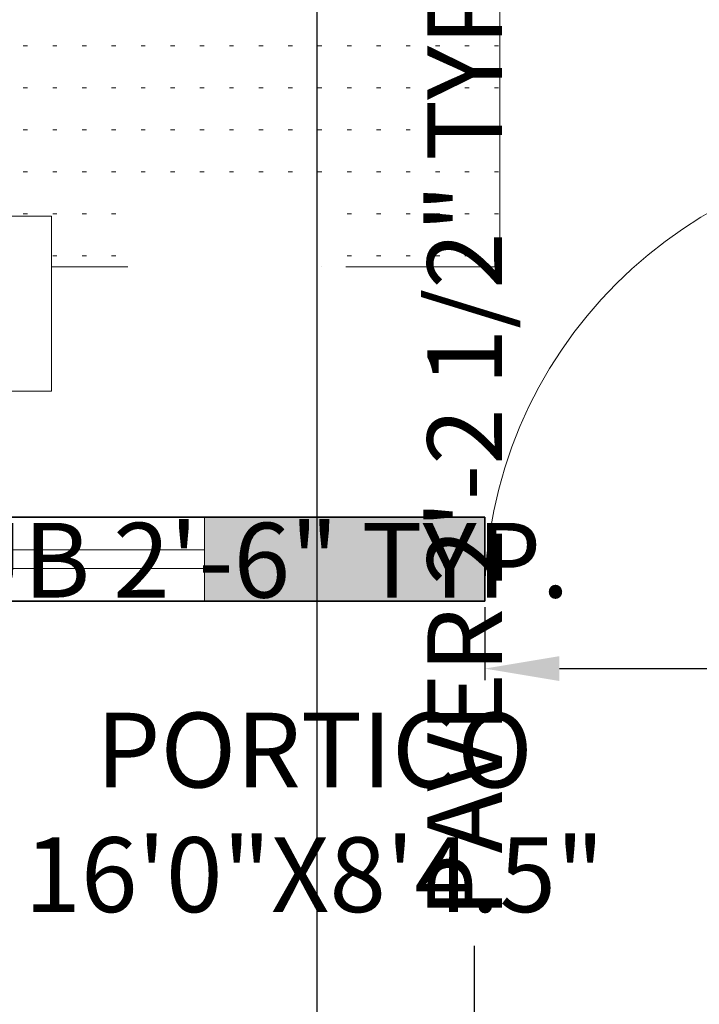
# Model space of a CAD drawing. Units: inches. Extents: x 2408 to 5087, y 2429 to 5085.
# Tile 5 of 12: x 2564 to 2636, y 2570 to 2676. Entities that reach past the tile are written whole.
import ezdxf

# ---------------------------------------------------------------- set-up
doc = ezdxf.new("R2010")
doc.units = ezdxf.units.IN
for name, color, linetype, lineweight in [('A-ANNO-DIMS', 2, 'Continuous', 18), ('A-AREA-IDEN', 6, 'Continuous', 18), ('A-DOOR', 3, 'Continuous', 18), ('A-FLOR-PATT', 8, 'Continuous', 13), ('A-FURN', 72, 'Continuous', 18), ('A-GLAZ', 4, 'Continuous', 18), ('A-WALL', 7, 'Continuous', 35), ('A-WALL-PATT', 252, 'Continuous', 13)]:
    doc.layers.add(name, color=color, linetype=linetype, lineweight=lineweight)
doc.styles.get("Standard").update_dxf_attribs({"font": 'arial.ttf'})
doc.dimstyles.new('ISO-25', dxfattribs={"dimtxt": 8, "dimasz": 8, "dimexe": 1.25, "dimexo": 0.625, "dimtad": 0, "dimdec": 1, "dimlunit": 4, "dimtxsty": 'Standard', "dimcen": 2.5, "dimadec": 0, "dimazin": 0, "dimtfac": 1, "dimtdec": 1, "dimtmove": 0, "dimatfit": 3, "dimfxl": 1, "dimarcsym": 0})

# ---------------------------------------------------------------- blocks, each defined once
blk = doc.blocks.new('door')
blk.add_lwpolyline([(2353.246, 2862.233), (2353.246, 2898.06), (2351.474, 2898.06), (2351.474, 2862.233), (2353.246, 2862.233)])
blk.add_arc((2353.246, 2862.233), 35.827, 90, 180)
blk = doc.blocks.new('Clinicians and patient chairs 25_dwgmodels.com')
at = {"color": 0}
for points in [[(-289.5, -1.5, 0, 0, 0), (-290.1, -3.2, 4.37, 4.37, 0)], [(-287.1, -0.3, 0, 0, 0), (-289.5, -1.5, 4.37, 4.37, 0)], [(-287.1, -0.3, 0, 0, 0), (-265.1, -0.9, 4.37, 4.37, 0)], [(-265.1, -0.9, 0, 0, 0), (-198.5, -0.4, 4.37, 4.37, 0)], [(-198.5, -0.4, 0, 0, 0), (-92.3, -0.3, 4.37, 4.37, 0)], [(-92.3, -0.3, 0, 0, 0), (0, 0, 4.37, 4.37, 0)], [(92.3, -0.3, 0, 0, 0), (0, 0, 4.37, 4.37, 0)], [(198.5, -0.4, 0, 0, 0), (92.3, -0.3, 4.37, 4.37, 0)], [(265.7, -0.9, 0, 0, 0), (198.5, -0.4, 4.37, 4.37, 0)], [(287.7, -0.3, 0, 0, 0), (265.7, -0.9, 4.37, 4.37, 0)], [(287.7, -0.3, 0, 0, 0), (290.1, -1.5, 4.37, 4.37, 0)], [(290.1, -1.5, 0, 0, 0), (290.7, -3.2, 4.37, 4.37, 0)], [(-371.8, -16.6, 0, 0, 0), (-369.1, -9.1, 4.37, 4.37, 0)], [(-371.8, -16.5, 0, 0, 0), (-369.8, -11, 4.37, 4.37, 0)], [(-371.8, -16.6, 0, 0, 0), (-371.8, -705.5, 4.37, 4.37, 0)], [(-371.8, -16.6, 0, 0, 0), (-371.8, -705.5, 4.37, 4.37, 0)], [(-369.8, -8.3, 0, 0, 0), (-369.7, -10.5, 4.37, 4.37, 0)], [(-369.8, -8.3, 0, 0, 0), (-369.8, -9.6, 4.37, 4.37, 0)], [(-369.8, -8.3, 0, 0, 0), (-367.7, -8.5, 4.37, 4.37, 0)], [(-369.8, -11, 0, 0, 0), (-369.8, -11, 4.37, 4.37, 0)], [(-369.8, -11, 0, 0, 0), (-369.8, -11, 4.37, 4.37, 0)], [(-369.8, -11, 0, 0, 0), (-369.8, -11, 4.37, 4.37, 0)], [(-369.7, -10.5, 0, 0, 0), (-369.6, -10.6, 4.37, 4.37, 0)], [(-369.1, -9.1, 0, 0, 0), (-361.2, -6.5, 4.37, 4.37, 0)], [(-367.7, -8.5, 0, 0, 0), (-367.6, -8.6, 4.37, 4.37, 0)], [(-367.7, -8.5, 0, 0, 0), (-367.6, -8.6, 4.37, 4.37, 0)], [(-361.2, -6.5, 0, 0, 0), (-367.2, -8.4, 4.37, 4.37, 0)], [(-367.2, -8.4, 0, 0, 0), (-367.2, -8.4, 4.37, 4.37, 0)], [(-367.2, -8.5, 0, 0, 0), (-367.2, -8.4, 4.37, 4.37, 0)], [(-299.5, -6.5, 0, 0, 0), (-361.2, -6.5, 4.37, 4.37, 0)], [(-299.5, -6.5, 0, 0, 0), (-294.7, -8, 4.37, 4.37, 0)], [(-299.5, -6.5, 0, 0, 0), (-294.7, -8.1, 4.37, 4.37, 0)], [(-294.8, -48.3, 0, 0, 0), (-294.8, -31.9, 4.37, 4.37, 0)], [(-294.7, -6.7, 0, 0, 0), (-291.8, -2.6, 4.37, 4.37, 0)], [(-294.8, -31.9, 0, 0, 0), (-294.7, -6.7, 4.37, 4.37, 0)], [(-294.7, -29.9, 0, 0, 0), (-294.5, -13.6, 4.37, 4.37, 0)], [(-294.7, -29.9, 0, 0, 0), (-294.8, -31.9, 4.37, 4.37, 0)], [(-291.8, -2.6, 0, 0, 0), (-290.1, -3.2, 4.37, 4.37, 0)], [(-289.7, -10.8, 0, 0, 0), (-290.1, -3.2, 4.37, 4.37, 0)], [(-290.1, -51.3, 0, 0, 0), (-290, -30, 4.37, 4.37, 0)], [(-290, -30, 0, 0, 0), (-289.7, -10.8, 4.37, 4.37, 0)], [(290.3, -10.8, 0, 0, 0), (290.7, -3.2, 4.37, 4.37, 0)], [(290.7, -30, 0, 0, 0), (290.3, -10.8, 4.37, 4.37, 0)], [(292.4, -2.6, 0, 0, 0), (290.7, -3.2, 4.37, 4.37, 0)], [(290.7, -51.3, 0, 0, 0), (290.7, -30, 4.37, 4.37, 0)], [(295.4, -6.7, 0, 0, 0), (292.4, -2.6, 4.37, 4.37, 0)], [(295.4, -29.9, 0, 0, 0), (295.1, -13.6, 4.37, 4.37, 0)], [(299.5, -6.5, 0, 0, 0), (295.4, -7.9, 4.37, 4.37, 0)], [(299.5, -6.5, 0, 0, 0), (295.4, -7.8, 4.37, 4.37, 0)], [(295.4, -31.9, 0, 0, 0), (295.4, -6.7, 4.37, 4.37, 0)], [(295.4, -29.9, 0, 0, 0), (295.4, -31.9, 4.37, 4.37, 0)], [(295.4, -31.9, 0, 0, 0), (295.4, -48.3, 4.37, 4.37, 0)], [(299.5, -6.5, 0, 0, 0), (361.2, -6.5, 4.37, 4.37, 0)], [(369.1, -9.1, 0, 0, 0), (361.2, -6.5, 4.37, 4.37, 0)], [(369.1, -9.1, 0, 0, 0), (361.2, -6.5, 4.37, 4.37, 0)], [(361.2, -6.6, 0, 0, 0), (367.2, -8.4, 4.37, 4.37, 0)], [(367.2, -8.4, 0, 0, 0), (367.2, -8.4, 4.37, 4.37, 0)], [(367.2, -8.5, 0, 0, 0), (367.2, -8.4, 4.37, 4.37, 0)], [(367.7, -8.5, 0, 0, 0), (367.6, -8.6, 4.37, 4.37, 0)], [(367.7, -8.5, 0, 0, 0), (367.6, -8.6, 4.37, 4.37, 0)], [(369.8, -8.3, 0, 0, 0), (367.7, -8.5, 4.37, 4.37, 0)], [(371.8, -16.6, 0, 0, 0), (369.1, -9.1, 4.37, 4.37, 0)], [(369.4, -10, 0, 0, 0), (369.4, -10, 4.37, 4.37, 0)], [(369.7, -10.5, 0, 0, 0), (369.6, -10.6, 4.37, 4.37, 0)], [(369.8, -8.3, 0, 0, 0), (369.7, -10.5, 4.37, 4.37, 0)], [(369.8, -8.3, 0, 0, 0), (369.8, -9.6, 4.37, 4.37, 0)], [(371.8, -16.5, 0, 0, 0), (369.8, -11, 4.37, 4.37, 0)], [(369.8, -11, 0, 0, 0), (369.8, -11, 4.37, 4.37, 0)], [(369.8, -11, 0, 0, 0), (369.8, -11, 4.37, 4.37, 0)], [(369.8, -11, 0, 0, 0), (369.8, -11, 4.37, 4.37, 0)], [(371.8, -16.6, 0, 0, 0), (371.8, -705.5, 4.37, 4.37, 0)], [(-371.8, -44.1, 0, 0, 0), (-371.8, -361, 4.37, 4.37, 0)], [(-294.8, -48.3, 0, 0, 0), (-294.7, -60.2, 4.37, 4.37, 0)], [(-294.7, -60.2, 0, 0, 0), (-294.7, -69.9, 4.37, 4.37, 0)], [(-290, -64.7, 0, 0, 0), (-290.1, -51.3, 4.37, 4.37, 0)], [(-290, -64.7, 0, 0, 0), (-290, -74.5, 4.37, 4.37, 0)], [(-284.2, -72.8, 0, 0, 0), (-262.5, -66.3, 4.37, 4.37, 0)], [(-276.4, -68.7, 0, 0, 0), (-280.9, -71.1, 4.37, 4.37, 0)], [(-276.4, -68.7, 0, 0, 0), (-257.9, -63.2, 4.37, 4.37, 0)], [(-262.5, -66.3, 0, 0, 0), (-233.5, -62.8, 4.37, 4.37, 0)], [(-262, -69.5, 0, 0, 0), (-233.2, -66.1, 4.37, 4.37, 0)], [(-257.9, -63.2, 0, 0, 0), (-233.1, -60.2, 4.37, 4.37, 0)], [(-233.5, -62.8, 0, 0, 0), (-96.6, -62.8, 4.37, 4.37, 0)], [(-96.6, -66, 0, 0, 0), (-233.2, -66.1, 4.37, 4.37, 0)], [(-233.1, -60.2, 0, 0, 0), (-96.5, -60.1, 4.37, 4.37, 0)], [(126.5, -62.8, 0, 0, 0), (-96.6, -62.8, 4.37, 4.37, 0)], [(126.5, -66, 0, 0, 0), (-96.6, -66, 4.37, 4.37, 0)], [(126.4, -60.1, 0, 0, 0), (-96.5, -60.1, 4.37, 4.37, 0)], [(233.6, -60.2, 0, 0, 0), (126.4, -60.1, 4.37, 4.37, 0)], [(234, -62.8, 0, 0, 0), (126.5, -62.8, 4.37, 4.37, 0)], [(126.5, -66, 0, 0, 0), (233.8, -66.1, 4.37, 4.37, 0)], [(258.5, -63.2, 0, 0, 0), (233.6, -60.2, 4.37, 4.37, 0)], [(262.5, -69.5, 0, 0, 0), (233.8, -66.1, 4.37, 4.37, 0)], [(234, -62.8, 0, 0, 0), (263.1, -66.3, 4.37, 4.37, 0)], [(277, -68.7, 0, 0, 0), (258.5, -63.2, 4.37, 4.37, 0)], [(284.7, -72.8, 0, 0, 0), (263.1, -66.3, 4.37, 4.37, 0)], [(277, -68.7, 0, 0, 0), (281.4, -71.1, 4.37, 4.37, 0)], [(290.7, -64.7, 0, 0, 0), (290.7, -51.3, 4.37, 4.37, 0)], [(290.6, -74.5, 0, 0, 0), (290.7, -64.7, 4.37, 4.37, 0)], [(295.4, -60.2, 0, 0, 0), (295.4, -48.3, 4.37, 4.37, 0)], [(295.4, -60.2, 0, 0, 0), (295.4, -69.9, 4.37, 4.37, 0)], [(371.8, -44.1, 0, 0, 0), (371.8, -361, 4.37, 4.37, 0)], [(-293, -92.7, 0, 0, 0), (-295.9, -118.4, 4.37, 4.37, 0)], [(-294.7, -69.9, 0, 0, 0), (-294.7, -86.3, 4.37, 4.37, 0)], [(-294.7, -86.3, 0, 0, 0), (-294.7, -87.6, 4.37, 4.37, 0)], [(-294.7, -87.6, 0, 0, 0), (-294.7, -87.7, 4.37, 4.37, 0)], [(-294.5, -88.2, 0, 0, 0), (-294.7, -87.7, 4.37, 4.37, 0)], [(-292.8, -91.5, 0, 0, 0), (-294.5, -88.2, 4.37, 4.37, 0)], [(-293, -92.7, 0, 0, 0), (-291.6, -83.8, 4.37, 4.37, 0)], [(-291.8, -79.4, 0, 0, 0), (-284.2, -72.8, 4.37, 4.37, 0)], [(-291.8, -79.4, 0, 0, 0), (-291.8, -84.9, 4.37, 4.37, 0)], [(-291.6, -83.8, 0, 0, 0), (-290.8, -82.4, 4.37, 4.37, 0)], [(-283.3, -75.9, 0, 0, 0), (-290.8, -82.4, 4.37, 4.37, 0)], [(-290, -74.5, 0, 0, 0), (-290, -77.9, 4.37, 4.37, 0)], [(-283.3, -75.9, 0, 0, 0), (-262, -69.5, 4.37, 4.37, 0)], [(-280.9, -71.1, 0, 0, 0), (-282.2, -72.2, 4.37, 4.37, 0)], [(262.5, -69.5, 0, 0, 0), (283.8, -75.9, 4.37, 4.37, 0)], [(281.4, -71.1, 0, 0, 0), (282.8, -72.2, 4.37, 4.37, 0)], [(283.8, -75.9, 0, 0, 0), (289.6, -80.9, 4.37, 4.37, 0)], [(284.7, -72.8, 0, 0, 0), (291.2, -78.5, 4.37, 4.37, 0)], [(289.8, -81.8, 0, 0, 0), (289.6, -80.9, 4.37, 4.37, 0)], [(289.8, -81.8, 0, 0, 0), (291.4, -92.3, 4.37, 4.37, 0)], [(290.6, -74.5, 0, 0, 0), (290.7, -78, 4.37, 4.37, 0)], [(292.4, -98.2, 0, 0, 0), (291.2, -78.5, 4.37, 4.37, 0)], [(294.4, -118.8, 0, 0, 0), (291.4, -92.3, 4.37, 4.37, 0)], [(292.1, -93.2, 0, 0, 0), (292.6, -93.1, 4.37, 4.37, 0)], [(292.3, -100.4, 0, 0, 0), (292.4, -100.3, 4.37, 4.37, 0)], [(292.4, -100.2, 0, 0, 0), (292.4, -98.2, 4.37, 4.37, 0)], [(292.8, -92.7, 0, 0, 0), (292.6, -93.1, 4.37, 4.37, 0)], [(292.8, -92.7, 0, 0, 0), (294.5, -89.3, 4.37, 4.37, 0)], [(294.5, -89.3, 0, 0, 0), (294.9, -88.5, 4.37, 4.37, 0)], [(294.9, -88.5, 0, 0, 0), (295.3, -87.6, 4.37, 4.37, 0)], [(295.4, -69.9, 0, 0, 0), (295.3, -86.3, 4.37, 4.37, 0)], [(295.3, -86.3, 0, 0, 0), (295.3, -87.8, 4.37, 4.37, 0)], [(-295.9, -118.4, 0, 0, 0), (-295.9, -139.7, 4.37, 4.37, 0)], [(294.4, -118.8, 0, 0, 0), (296.4, -139.7, 4.37, 4.37, 0)], [(-295.9, -139.7, 0, 0, 0), (-295.9, -144.1, 4.37, 4.37, 0)], [(-295.6, -147.4, 0, 0, 0), (-295.9, -144.1, 4.37, 4.37, 0)], [(-295.6, -147.4, 0, 0, 0), (-294.9, -155.8, 4.37, 4.37, 0)], [(-294.9, -155.8, 0, 0, 0), (-294, -165.2, 4.37, 4.37, 0)], [(-294, -165.2, 0, 0, 0), (-293.2, -174.7, 4.37, 4.37, 0)], [(-292.1, -160, 0, 0, 0), (-291, -157.5, 4.37, 4.37, 0)], [(-292.1, -182.8, 0, 0, 0), (-292.1, -160, 4.37, 4.37, 0)], [(-283.4, -148.6, 0, 0, 0), (-291, -157.5, 4.37, 4.37, 0)], [(-289, -161.1, 0, 0, 0), (-289.1, -183.8, 4.37, 4.37, 0)], [(-288.7, -160.4, 0, 0, 0), (-289, -161.1, 4.37, 4.37, 0)], [(-283.4, -148.6, 0, 0, 0), (-262.3, -142.9, 4.37, 4.37, 0)], [(-261.4, -146.5, 0, 0, 0), (-282, -152.1, 4.37, 4.37, 0)], [(-261.8, -142.8, 0, 0, 0), (-262.3, -142.9, 4.37, 4.37, 0)], [(-261.4, -146.5, 0, 0, 0), (-233.4, -145.3, 4.37, 4.37, 0)], [(-233.4, -145.3, 0, 0, 0), (-96.7, -145.6, 4.37, 4.37, 0)], [(-96.7, -145.6, 0, 0, 0), (126.7, -145.6, 4.37, 4.37, 0)], [(233.9, -145.3, 0, 0, 0), (126.7, -145.6, 4.37, 4.37, 0)], [(261.9, -146.5, 0, 0, 0), (233.9, -145.3, 4.37, 4.37, 0)], [(261.9, -146.5, 0, 0, 0), (282.5, -152.1, 4.37, 4.37, 0)], [(262.4, -142.8, 0, 0, 0), (262.8, -142.9, 4.37, 4.37, 0)], [(283.9, -148.6, 0, 0, 0), (262.8, -142.9, 4.37, 4.37, 0)], [(283.9, -148.6, 0, 0, 0), (291.5, -157.5, 4.37, 4.37, 0)], [(289.2, -160.4, 0, 0, 0), (289.6, -161.1, 4.37, 4.37, 0)], [(289.6, -161.1, 0, 0, 0), (289.6, -183.8, 4.37, 4.37, 0)], [(292.6, -160, 0, 0, 0), (291.5, -157.5, 4.37, 4.37, 0)], [(292.6, -160, 0, 0, 0), (292.7, -182.8, 4.37, 4.37, 0)], [(294.1, -170, 0, 0, 0), (294, -171.7, 4.37, 4.37, 0)], [(294.1, -170, 0, 0, 0), (294.9, -162, 4.37, 4.37, 0)], [(294.9, -162, 0, 0, 0), (296.2, -147, 4.37, 4.37, 0)], [(296.2, -147, 0, 0, 0), (296.4, -144.1, 4.37, 4.37, 0)], [(296.4, -139.7, 0, 0, 0), (296.4, -144.7, 4.37, 4.37, 0)], [(-292.1, -183.2, 0, 0, 0), (-293.2, -174.7, 4.37, 4.37, 0)], [(-292.1, -182.8, 0, 0, 0), (-292.1, -189.8, 4.37, 4.37, 0)], [(-291, -191.1, 0, 0, 0), (-292.1, -190.5, 4.37, 4.37, 0)], [(-290.4, -191.5, 0, 0, 0), (-291, -191.1, 4.37, 4.37, 0)], [(-290, -191.9, 0, 0, 0), (-290.4, -191.5, 4.37, 4.37, 0)], [(-290, -191.9, 0, 0, 0), (-289.4, -192.4, 4.37, 4.37, 0)], [(-289.1, -192.4, 0, 0, 0), (-289.4, -192.4, 4.37, 4.37, 0)], [(-289.1, -192.9, 0, 0, 0), (-289.1, -183.8, 4.37, 4.37, 0)], [(-288.9, -193.4, 0, 0, 0), (-289.1, -192.9, 4.37, 4.37, 0)], [(-288.9, -193.4, 0, 0, 0), (-288.9, -193.4, 4.37, 4.37, 0)], [(-288.9, -194.1, 0, 0, 0), (-288.9, -686.6, 4.37, 4.37, 0)], [(-288.9, -197.7, 0, 0, 0), (-288.9, -361, 4.37, 4.37, 0)], [(-288.9, -197.7, 0, 0, 0), (-288.9, -686.6, 4.37, 4.37, 0)], [(289.5, -193, 0, 0, 0), (288.9, -194.6, 4.37, 4.37, 0)], [(288.9, -194.1, 0, 0, 0), (288.9, -686.6, 4.37, 4.37, 0)], [(288.9, -199.4, 0, 0, 0), (288.9, -361, 4.37, 4.37, 0)], [(289.5, -193, 0, 0, 0), (289.6, -192.6, 4.37, 4.37, 0)], [(289.6, -183.8, 0, 0, 0), (289.6, -191.3, 4.37, 4.37, 0)], [(289.8, -192.1, 0, 0, 0), (289.6, -192, 4.37, 4.37, 0)], [(289.8, -192.1, 0, 0, 0), (290, -192.1, 4.37, 4.37, 0)], [(290.4, -191.7, 0, 0, 0), (290, -192.1, 4.37, 4.37, 0)], [(290.5, -191.6, 0, 0, 0), (291, -191.2, 4.37, 4.37, 0)], [(290.5, -191.6, 0, 0, 0), (290.4, -191.7, 4.37, 4.37, 0)], [(291, -191.2, 0, 0, 0), (292.7, -190.4, 4.37, 4.37, 0)], [(292.7, -183.1, 0, 0, 0), (293.7, -174.6, 4.37, 4.37, 0)], [(292.7, -182.8, 0, 0, 0), (292.7, -189.8, 4.37, 4.37, 0)], [(294, -171.7, 0, 0, 0), (293.7, -174.6, 4.37, 4.37, 0)], [(-288.3, -246.3, 0, 0, 0), (-288.9, -245.1, 4.37, 4.37, 0)], [(-286.9, -248.4, 0, 0, 0), (-288.9, -247.9, 4.37, 4.37, 0)], [(-288.3, -246.3, 0, 0, 0), (-286, -249.9, 4.37, 4.37, 0)], [(-281.3, -252.3, 0, 0, 0), (-286, -249.9, 4.37, 4.37, 0)], [(-281.3, -252.3, 0, 0, 0), (-276, -253.6, 4.37, 4.37, 0)], [(-276, -253.6, 0, 0, 0), (-230.3, -254.3, 4.37, 4.37, 0)], [(-230.3, -254.3, 0, 0, 0), (-94.3, -254.3, 4.37, 4.37, 0)], [(124.3, -254.3, 0, 0, 0), (-94.3, -254.3, 4.37, 4.37, 0)], [(230.8, -254.3, 0, 0, 0), (124.3, -254.3, 4.37, 4.37, 0)], [(276.5, -253.6, 0, 0, 0), (230.8, -254.3, 4.37, 4.37, 0)], [(281.8, -252.3, 0, 0, 0), (276.5, -253.6, 4.37, 4.37, 0)], [(281.8, -252.3, 0, 0, 0), (286.5, -249.9, 4.37, 4.37, 0)], [(286.5, -249.9, 0, 0, 0), (288.9, -246.3, 4.37, 4.37, 0)], [(287.5, -248.4, 0, 0, 0), (288.9, -248, 4.37, 4.37, 0)], [(288.9, -246.3, 0, 0, 0), (288.9, -246.2, 4.37, 4.37, 0)], [(-371.8, -705.5, 0, 0, 0), (-371.8, -361, 4.37, 4.37, 0)], [(-288.9, -705.5, 0, 0, 0), (-288.9, -361, 4.37, 4.37, 0)], [(288.9, -686.6, 0, 0, 0), (288.9, -361, 4.37, 4.37, 0)], [(371.8, -705.5, 0, 0, 0), (371.8, -361, 4.37, 4.37, 0)], [(-371.8, -705.5, 0, 0, 0), (-369.8, -711.1, 4.37, 4.37, 0)], [(-371.8, -705.5, 0, 0, 0), (-369.1, -713, 4.37, 4.37, 0)], [(-288.9, -705.5, 0, 0, 0), (-291.6, -713, 4.37, 4.37, 0)], [(-288.9, -705.5, 0, 0, 0), (-291.6, -713, 4.37, 4.37, 0)], [(-288.9, -705.5, 0, 0, 0), (-290.9, -711.1, 4.37, 4.37, 0)], [(-288.9, -686.9, 0, 0, 0), (-288.9, -705.5, 4.37, 4.37, 0)], [(-288.9, -686.9, 0, 0, 0), (-288.9, -705.5, 4.37, 4.37, 0)], [(288.9, -686.9, 0, 0, 0), (288.9, -705.5, 4.37, 4.37, 0)], [(288.9, -705.5, 0, 0, 0), (288.9, -686.9, 4.37, 4.37, 0)], [(288.9, -705.5, 0, 0, 0), (291.6, -713, 4.37, 4.37, 0)], [(288.9, -705.5, 0, 0, 0), (291.6, -713, 4.37, 4.37, 0)], [(288.9, -705.5, 0, 0, 0), (290.9, -711.1, 4.37, 4.37, 0)], [(371.8, -705.5, 0, 0, 0), (369.1, -713, 4.37, 4.37, 0)], [(371.8, -705.5, 0, 0, 0), (369.1, -713, 4.37, 4.37, 0)], [(371.8, -705.5, 0, 0, 0), (369.8, -711.1, 4.37, 4.37, 0)], [(-369.8, -711.1, 0, 0, 0), (-369.8, -711.1, 4.37, 4.37, 0)], [(-369.8, -711.1, 0, 0, 0), (-369.8, -711.1, 4.37, 4.37, 0)], [(-369.8, -713.8, 0, 0, 0), (-369.7, -711.6, 4.37, 4.37, 0)], [(-369.8, -713.8, 0, 0, 0), (-367.7, -713.6, 4.37, 4.37, 0)], [(-369.8, -713.8, 0, 0, 0), (-368.6, -713.7, 4.37, 4.37, 0)], [(-369.7, -711.6, 0, 0, 0), (-369.7, -711.5, 4.37, 4.37, 0)], [(-369.3, -712.5, 0, 0, 0), (-369.2, -712.7, 4.37, 4.37, 0)], [(-369.2, -712.7, 0, 0, 0), (-369.2, -712.8, 4.37, 4.37, 0)], [(-369.1, -713, 0, 0, 0), (-361.2, -715.5, 4.37, 4.37, 0)], [(-367.7, -713.6, 0, 0, 0), (-367.6, -713.5, 4.37, 4.37, 0)], [(-367.7, -713.6, 0, 0, 0), (-367.6, -713.5, 4.37, 4.37, 0)], [(-367.2, -713.7, 0, 0, 0), (-367.2, -713.6, 4.37, 4.37, 0)], [(-367.2, -713.6, 0, 0, 0), (-367.2, -713.6, 4.37, 4.37, 0)], [(-361.2, -715.5, 0, 0, 0), (-367.2, -713.7, 4.37, 4.37, 0)], [(-361.2, -715.5, 0, 0, 0), (-299.5, -715.5, 4.37, 4.37, 0)], [(-299.5, -715.5, 0, 0, 0), (-361.2, -715.5, 4.37, 4.37, 0)], [(-299.5, -715.5, 0, 0, 0), (-291.6, -713, 4.37, 4.37, 0)], [(-299.5, -715.5, 0, 0, 0), (-293.5, -713.7, 4.37, 4.37, 0)], [(-294.3, -713.9, 0, 0, 0), (-291.6, -721.7, 4.37, 4.37, 0)], [(-293, -713.6, 0, 0, 0), (-293.1, -713.5, 4.37, 4.37, 0)], [(-290.8, -713.8, 0, 0, 0), (-293, -713.6, 4.37, 4.37, 0)], [(-291.4, -721.7, 0, 0, 0), (-291.6, -721.7, 4.37, 4.37, 0)], [(-291.5, -713.7, 0, 0, 0), (-291.5, -715.5, 4.37, 4.37, 0)], [(-291.4, -721.7, 0, 0, 0), (-291.5, -715.5, 4.37, 4.37, 0)], [(-291.4, -722.2, 0, 0, 0), (-291.4, -721.7, 4.37, 4.37, 0)], [(-290.2, -724.2, 0, 0, 0), (-291.4, -722.2, 4.37, 4.37, 0)], [(-290.9, -711.6, 0, 0, 0), (-291, -711.5, 4.37, 4.37, 0)], [(-290.9, -713.8, 0, 0, 0), (-290.9, -711.6, 4.37, 4.37, 0)], [(-290.8, -713.8, 0, 0, 0), (-290.9, -712.4, 4.37, 4.37, 0)], [(-290.2, -724.2, 0, 0, 0), (-287.9, -724.4, 4.37, 4.37, 0)], [(-287.6, -723.9, 0, 0, 0), (-287.9, -724.4, 4.37, 4.37, 0)], [(-287.6, -723.9, 0, 0, 0), (-287.4, -724.4, 4.37, 4.37, 0)], [(-281.6, -725.6, 0, 0, 0), (-287.4, -724.4, 4.37, 4.37, 0)], [(-232.7, -728.2, 0, 0, 0), (-281.6, -725.3, 4.37, 4.37, 0)], [(-281.6, -725.6, 0, 0, 0), (-259.9, -726.6, 4.37, 4.37, 0)], [(-232.7, -728.2, 0, 0, 0), (-175.7, -728.3, 4.37, 4.37, 0)], [(-85.2, -724.6, 0, 0, 0), (-175.7, -728.3, 4.37, 4.37, 0)], [(-85.2, -724.6, 0, 0, 0), (0, -724.8, 4.37, 4.37, 0)], [(0, -724.8, 0, 0, 0), (85.2, -724.6, 4.37, 4.37, 0)], [(85.2, -724.6, 0, 0, 0), (175.7, -728.3, 4.37, 4.37, 0)], [(232.7, -728.2, 0, 0, 0), (175.7, -728.3, 4.37, 4.37, 0)], [(232.7, -728.2, 0, 0, 0), (281.6, -725.3, 4.37, 4.37, 0)], [(259.9, -726.6, 0, 0, 0), (281.6, -725.6, 4.37, 4.37, 0)], [(281.6, -725.6, 0, 0, 0), (287.4, -724.4, 4.37, 4.37, 0)], [(287.4, -724.4, 0, 0, 0), (287.6, -723.9, 4.37, 4.37, 0)], [(287.9, -724.4, 0, 0, 0), (287.6, -723.9, 4.37, 4.37, 0)], [(290.2, -724.2, 0, 0, 0), (287.9, -724.4, 4.37, 4.37, 0)], [(291.4, -722.2, 0, 0, 0), (290.2, -724.2, 4.37, 4.37, 0)], [(290.9, -713.8, 0, 0, 0), (290.9, -711.6, 4.37, 4.37, 0)], [(290.8, -713.8, 0, 0, 0), (290.9, -712.4, 4.37, 4.37, 0)], [(290.8, -713.8, 0, 0, 0), (293, -713.6, 4.37, 4.37, 0)], [(290.9, -711.6, 0, 0, 0), (291, -711.5, 4.37, 4.37, 0)], [(291.4, -721.7, 0, 0, 0), (291.5, -715.5, 4.37, 4.37, 0)], [(291.6, -721.7, 0, 0, 0), (291.4, -721.7, 4.37, 4.37, 0)], [(291.4, -722.2, 0, 0, 0), (291.4, -721.7, 4.37, 4.37, 0)], [(291.5, -713.7, 0, 0, 0), (291.5, -715.5, 4.37, 4.37, 0)], [(299.5, -715.5, 0, 0, 0), (291.6, -713, 4.37, 4.37, 0)], [(294.3, -713.9, 0, 0, 0), (291.6, -721.7, 4.37, 4.37, 0)], [(293, -713.6, 0, 0, 0), (293.1, -713.5, 4.37, 4.37, 0)], [(299.5, -715.5, 0, 0, 0), (293.5, -713.7, 4.37, 4.37, 0)], [(299.5, -715.5, 0, 0, 0), (361.2, -715.5, 4.37, 4.37, 0)], [(299.5, -715.5, 0, 0, 0), (361.2, -715.5, 4.37, 4.37, 0)], [(299.5, -715.5, 0, 0, 0), (361.2, -715.5, 4.37, 4.37, 0)], [(361.2, -715.5, 0, 0, 0), (299.5, -715.5, 4.37, 4.37, 0)], [(369.1, -713, 0, 0, 0), (361.2, -715.5, 4.37, 4.37, 0)], [(369.1, -713, 0, 0, 0), (361.2, -715.5, 4.37, 4.37, 0)], [(361.2, -715.5, 0, 0, 0), (367.2, -713.7, 4.37, 4.37, 0)], [(367.2, -713.6, 0, 0, 0), (367.2, -713.6, 4.37, 4.37, 0)], [(367.2, -713.7, 0, 0, 0), (367.2, -713.6, 4.37, 4.37, 0)], [(367.7, -713.6, 0, 0, 0), (367.6, -713.5, 4.37, 4.37, 0)], [(367.7, -713.6, 0, 0, 0), (367.6, -713.5, 4.37, 4.37, 0)], [(369.8, -713.8, 0, 0, 0), (367.7, -713.6, 4.37, 4.37, 0)], [(369.8, -713.8, 0, 0, 0), (368.7, -713.7, 4.37, 4.37, 0)], [(369.7, -711.6, 0, 0, 0), (369.7, -711.5, 4.37, 4.37, 0)], [(369.8, -711.1, 0, 0, 0), (369.8, -711.1, 4.37, 4.37, 0)], [(369.8, -711.1, 0, 0, 0), (369.8, -711.1, 4.37, 4.37, 0)], [(369.8, -713.8, 0, 0, 0), (369.7, -711.6, 4.37, 4.37, 0)]]:
    blk.add_lwpolyline(points, format="xyseb", dxfattribs=at)
blk = doc.blocks.new('WIN-60x9')
for p, q in [((3.5, 60), (3.5, 0)), ((5.5, 60), (5.5, 0))]:
    blk.add_line(p, q)
blk.add_lwpolyline([(0, 60), (9, 60), (9, 0), (0, 0)], close=True)
blk = doc.blocks.new('*D27')
at = {"layer": 'A-ANNO-DIMS', "color": 0, "lineweight": -2, "transparency": 16777216}
for p, q in [((2612.36, 2568.68), (2612.36, 2576.68)), ((2608.98, 2568.68), (2613.61, 2568.68)), ((2612.36, 2550.04), (2612.36, 2560.68)), ((2608.98, 2542.04), (2613.61, 2542.04))]:
    blk.add_line(p, q, dxfattribs=at)
at = {"layer": 'A-ANNO-DIMS', "color": 0, "transparency": 16777216}
for points in [[(2611.02, 2560.68), (2613.69, 2560.68), (2612.36, 2568.68)], [(2611.02, 2550.04), (2613.69, 2550.04), (2612.36, 2542.04)]]:
    blk.add_solid(points, dxfattribs=at)
at = {"layer": 'Defpoints', "color": 0, "transparency": 16777216}
for p in [(2608.36, 2568.68), (2612.36, 2568.68), (2608.36, 2542.04)]:
    blk.add_point(p, dxfattribs=at)
at = {"layer": 'A-ANNO-DIMS', "color": 0, "transparency": 16777216, "insert": (2612.36, 2631.3), "char_height": 8, "attachment_point": 5, "rotation": 90}
blk.add_mtext('PAVER 2\'-2 1/2" TYP.', dxfattribs=at)
blk = doc.blocks.new('*D29')
at = {"layer": 'A-ANNO-DIMS', "color": 0, "lineweight": -2, "transparency": 16777216}
for p, q in [((2494.62, 2613.03), (2494.62, 2618.16)), ((2524.6, 2613.03), (2524.6, 2618.16)), ((2502.62, 2616.91), (2516.6, 2616.91)), ((2524.6, 2616.91), (2532.6, 2616.91))]:
    blk.add_line(p, q, dxfattribs=at)
at = {"layer": 'A-ANNO-DIMS', "color": 0, "transparency": 16777216}
for points in [[(2502.62, 2618.24), (2502.62, 2615.57), (2494.62, 2616.91)], [(2516.6, 2618.24), (2516.6, 2615.57), (2524.6, 2616.91)]]:
    blk.add_solid(points, dxfattribs=at)
at = {"layer": 'Defpoints', "color": 0, "transparency": 16777216}
for p in [(2524.6, 2616.91), (2494.62, 2612.41), (2524.6, 2612.41)]:
    blk.add_point(p, dxfattribs=at)
at = {"layer": 'A-ANNO-DIMS', "color": 0, "transparency": 16777216, "insert": (2578.7, 2616.91), "char_height": 8, "attachment_point": 5}
blk.add_mtext('SHRUB 2\'-6" TYP.', dxfattribs=at)
blk = doc.blocks.new('*D39')
at = {"layer": 'A-ANNO-DIMS', "color": 0, "lineweight": -2, "transparency": 16777216}
for p, q in [((2613.46, 2612.93), (2613.46, 2605.1)), ((2661.49, 2612.93), (2661.49, 2605.1)), ((2621.46, 2606.35), (2653.49, 2606.35)), ((2661.49, 2606.35), (2669.49, 2606.35))]:
    blk.add_line(p, q, dxfattribs=at)
at = {"layer": 'A-ANNO-DIMS', "color": 0, "transparency": 16777216}
for points in [[(2621.46, 2607.68), (2621.46, 2605.02), (2613.46, 2606.35)], [(2653.49, 2607.68), (2653.49, 2605.02), (2661.49, 2606.35)]]:
    blk.add_solid(points, dxfattribs=at)
at = {"layer": 'Defpoints', "color": 0, "transparency": 16777216}
for p in [(2613.46, 2613.55), (2661.49, 2613.55), (2661.49, 2606.35)]:
    blk.add_point(p, dxfattribs=at)
at = {"layer": 'A-ANNO-DIMS', "color": 0, "transparency": 16777216, "insert": (2698.87, 2606.35), "char_height": 8, "attachment_point": 5}
blk.add_mtext('DOOR 4\'-0"', dxfattribs=at)
blk = doc.blocks.new('*D61')
at = {"layer": 'A-ANNO-DIMS', "color": 0, "lineweight": -2, "transparency": 16777216}
for p, q in [((2493.49, 2813.93), (2493.49, 2439.55)), ((2595.49, 2813.93), (2595.49, 2439.55)), ((2501.49, 2440.8), (2533.23, 2440.8)), ((2587.49, 2440.8), (2555.76, 2440.8))]:
    blk.add_line(p, q, dxfattribs=at)
at = {"layer": 'A-ANNO-DIMS', "color": 0, "transparency": 16777216}
for points in [[(2501.49, 2442.13), (2501.49, 2439.47), (2493.49, 2440.8)], [(2587.49, 2442.13), (2587.49, 2439.47), (2595.49, 2440.8)]]:
    blk.add_solid(points, dxfattribs=at)
at = {"layer": 'Defpoints', "color": 0, "transparency": 16777216}
for p in [(2493.49, 2814.55), (2595.49, 2814.55), (2595.49, 2440.8)]:
    blk.add_point(p, dxfattribs=at)
at = {"layer": 'A-ANNO-DIMS', "color": 0, "transparency": 16777216, "insert": (2544.49, 2440.8), "char_height": 8, "attachment_point": 5}
blk.add_mtext('8\'-6"', dxfattribs=at)

msp = doc.modelspace()

# ---------------------------------------------------------------- hatches: boundary and pattern name
at = {"layer": 'A-FLOR-PATT'}
h = msp.add_hatch(dxfattribs=at)
h.set_pattern_fill('ACAD_ISO07W100', color=256, scale=0.9)
h.paths.add_polyline_path([(2562.5, 2700.89), (2556.3, 2700.89), (2556.3, 2686.85), (2562.5, 2686.85)], flags=0)
h.paths.add_polyline_path([(2615.08, 2748.91), (2506.63, 2748.91), (2506.63, 2731.92), (2517.79, 2731.92), (2518.12, 2731.8), (2518.26, 2731.5), (2518.24, 2731.53), (2518.24, 2668.18), (2517.9, 2667.99), (2506.63, 2667.99), (2506.63, 2649.35), (2525.6, 2649.35), (2525.6, 2656.74), (2525.67, 2656.76), (2525.66, 2656.79), (2525.7, 2656.79), (2525.74, 2656.78), (2525.93, 2656.85), (2525.94, 2656.85), (2528.05, 2656.85), (2528.14, 2657.1), (2528.15, 2657.1), (2528.16, 2657.12), (2528.24, 2657.12), (2528.43, 2657.16), (2529.11, 2657.19), (2529.97, 2657.24), (2531.76, 2657.24), (2534.59, 2657.13), (2537.27, 2657.14), (2539.94, 2657.13), (2542.78, 2657.24), (2544.57, 2657.24), (2545.42, 2657.19), (2546.38, 2657.15), (2546.5, 2656.79), (2546.66, 2656.85), (2548.6, 2656.85), (2548.82, 2656.85), (2548.84, 2656.79), (2548.87, 2656.79), (2548.87, 2656.71), (2548.96, 2656.45), (2548.93, 2656.53), (2548.93, 2649.35), (2556.54, 2649.35), (2556.54, 2654.76), (2567.14, 2654.76), (2567.14, 2649.35), (2575.28, 2649.35), (2575.28, 2656.74), (2575.34, 2656.76), (2575.34, 2656.79), (2575.38, 2656.79), (2575.42, 2656.78), (2575.61, 2656.85), (2575.61, 2656.85), (2577.73, 2656.85), (2577.82, 2657.1), (2577.83, 2657.1), (2577.84, 2657.12), (2577.92, 2657.12), (2578.11, 2657.16), (2578.79, 2657.19), (2579.64, 2657.24), (2581.43, 2657.24), (2584.27, 2657.13), (2586.94, 2657.14), (2589.62, 2657.13), (2592.46, 2657.24), (2594.25, 2657.24), (2595.1, 2657.19), (2596.05, 2657.15), (2596.18, 2656.79), (2596.34, 2656.85), (2598.28, 2656.85), (2598.5, 2656.85), (2598.52, 2656.79), (2598.55, 2656.79), (2598.55, 2656.71), (2598.64, 2656.45), (2598.61, 2656.53), (2598.61, 2649.35), (2615.08, 2649.35)])
h.paths.add_polyline_path([(2570.6, 2678.23), (2548.2, 2678.23), (2548.2, 2722.4), (2570.6, 2722.4)], flags=16)
h.paths.add_polyline_path([(2562.5, 2686.85), (2556.3, 2686.85), (2556.3, 2700.89), (2562.5, 2700.89)], flags=0)
at = {"layer": 'A-WALL-PATT'}
h = msp.add_hatch(color=256, dxfattribs=at)
h.dxf.hatch_style = 1
h.paths.add_polyline_path([(2493.49, 2613.55), (2523.49, 2613.55), (2523.49, 2622.55), (2493.49, 2622.55), (2493.49, 2714.8), (2484.49, 2714.8), (2484.49, 2497.75), (2493.49, 2497.75)])
h.paths.add_polyline_path([(2613.49, 2615.42), (2613.49, 2622.55), (2583.49, 2622.55), (2583.49, 2613.55), (2613.46, 2613.55, -0.009707)])
h.paths.add_polyline_path([(2823.49, 2634.55), (2814.49, 2634.55), (2814.49, 2622.55), (2694.49, 2622.55), (2694.49, 2670.55), (2706.49, 2670.55), (2706.49, 2675.05), (2694.49, 2675.05), (2694.49, 2750.05), (2685.49, 2750.05), (2685.49, 2622.55), (2661.49, 2622.55), (2661.49, 2613.55), (2814.49, 2613.55), (2814.49, 2522.05), (2688.49, 2522.05), (2688.49, 2513.05), (2823.49, 2513.05)])
h.paths.add_polyline_path([(2823.49, 2837.05), (2814.49, 2837.05), (2814.49, 2819.05), (2685.49, 2819.05), (2685.49, 2786.05), (2694.49, 2786.05), (2694.49, 2810.05), (2814.49, 2810.05), (2814.49, 2772.55), (2823.49, 2772.55)])
h.paths.add_polyline_path([(2694.49, 2964.55), (2595.49, 2964.55), (2595.49, 3008.05), (2601.49, 3008.05), (2601.49, 3017.05), (2484.49, 3017.05), (2484.49, 2972.05), (2493.49, 2972.05), (2493.49, 3008.05), (2586.49, 3008.05), (2586.49, 2955.55), (2685.49, 2955.55), (2685.49, 2854.87), (2694.49, 2854.87)])
h.paths.add_polyline_path([(2493.49, 2867.05), (2595.49, 2867.05), (2595.49, 2876.05), (2493.49, 2876.05), (2493.49, 2912.05), (2484.49, 2912.05), (2484.49, 2774.8), (2493.49, 2774.8)])
h.paths.add_polyline_path([(2595.49, 2814.55), (2493.49, 2814.55), (2493.49, 2810.05), (2595.49, 2810.05)], flags=17)
h.paths.add_polyline_path([(2724.49, 3017.05), (2625.49, 3017.05), (2625.49, 3008.05), (2685.49, 3008.05), (2685.49, 2994.55), (2694.49, 2994.55), (2694.49, 3008.05), (2724.49, 3008.05)])
h.paths.add_polyline_path([(2823.49, 3017.05), (2784.49, 3017.05), (2784.49, 3008.05), (2814.49, 3008.05), (2814.49, 2913.55), (2814.56, 2897.05), (2823.49, 2897.05)])
h.paths.add_polyline_path([(2823.49, 2712.55), (2814.61, 2712.55), (2814.66, 2701.27), (2814.49, 2701.27), (2814.49, 2675.05), (2740.99, 2675.05), (2740.99, 2687.05), (2736.49, 2687.05), (2736.49, 2670.55), (2814.49, 2670.55), (2814.49, 2658.55), (2823.49, 2658.55)], flags=17)

# ---------------------------------------------------------------- linework, layer by layer
at = {"layer": 'A-FURN'}
msp.add_line((2567.14, 2649.35), (2575.28, 2649.35), dxfattribs=at)
for points in [[(2598.61, 2649.35), (2615.08, 2649.35), (2615.08, 2748.91), (2506.63, 2748.91), (2506.63, 2731.84)], [(2596.01, 2649.35), (2596.01, 2649.35)]]:
    msp.add_lwpolyline(points, dxfattribs=at)
msp.add_lwpolyline([(2556.54, 2654.76), (2567.14, 2654.76), (2567.14, 2636.04), (2556.54, 2636.04)], close=True, dxfattribs=at)
at = {"layer": 'A-WALL'}
for p, q in [((2613.49, 2622.55), (2493.49, 2622.55)), ((2613.49, 2622.55), (2613.49, 2613.55)), ((2613.49, 2613.55), (2493.49, 2613.55))]:
    msp.add_line(p, q, dxfattribs=at)

# ---------------------------------------------------------------- block references
at = {"layer": 'A-DOOR', "xscale": 1.340790722123845, "yscale": 1.340790722123845, "zscale": 1.340790722123845}
msp.add_blockref('door', (-493.72, -1224.1), dxfattribs=at)
at = {"layer": 'A-FURN', "xscale": 0.0313747741943372, "yscale": 0.0313747741943372, "zscale": 0.0313747741943372, "rotation": 180}
msp.add_blockref('Clinicians and patient chairs 25_dwgmodels.com', (2586.94, 2634.4), dxfattribs=at)
at = {"layer": 'A-GLAZ', "rotation": 269.9999999999976}
msp.add_blockref('WIN-60x9', (2523.49, 2622.55), dxfattribs=at)

# ---------------------------------------------------------------- texts
at = {"layer": 'A-AREA-IDEN', "insert": (2543.8, 2601.63), "char_height": 8, "attachment_point": 1}
msp.add_mtext_dynamic_manual_height_columns('\\pxqc;PORTICO\\P16\'0"X8\'4.5"', width=102.8772, gutter_width=12.5, heights=[0], dxfattribs=at)

# ---------------------------------------------------------------- dimensions: what is measured, and where the dimension line sits
at = {"layer": 'A-ANNO-DIMS'}
dim = msp.add_linear_dim(base=(2595.49, 2440.8), p1=(2493.49, 2814.55), p2=(2595.49, 2814.55), dimstyle='ISO-25', override={"dimdec": 1, "dimlfac": 1, "dimrnd": 0, "dimzin": 1, "dimdsep": 46, "dimlunit": 4, "dimfrac": 2}, dxfattribs=at)
dim.commit()
dim.dimension.update_dxf_attribs({"geometry": '*D61', "text_midpoint": (2544.49, 2440.8)})
dim = msp.add_linear_dim(base=(2612.36, 2568.68), p1=(2608.36, 2542.04), p2=(2608.36, 2568.68), angle=90, text='PAVER <> TYP.', dimstyle='ISO-25', override={"dimdec": 1, "dimlfac": 1, "dimrnd": 0, "dimzin": 1, "dimdsep": 46, "dimlunit": 4, "dimfrac": 2}, dxfattribs=at)
dim.commit()
dim.dimension.update_dxf_attribs({"geometry": '*D27', "text_midpoint": (2612.36, 2631.3)})
for base, p1, p2, text, picture, middle in [((2524.6, 2616.91), (2494.62, 2612.41), (2524.6, 2612.41), 'SHRUB <> TYP.', '*D29', (2578.7, 2616.91)), ((2661.49, 2606.35), (2613.46, 2613.55), (2661.49, 2613.55), 'DOOR <>', '*D39', (2698.87, 2606.35))]:
    dim = msp.add_linear_dim(base=base, p1=p1, p2=p2, text=text, dimstyle='ISO-25', override={"dimdec": 1, "dimlfac": 1, "dimrnd": 0, "dimzin": 1, "dimdsep": 46, "dimlunit": 4, "dimfrac": 2}, dxfattribs=at)
    dim.commit()
    dim.dimension.update_dxf_attribs({"geometry": picture, "text_midpoint": middle})

doc.saveas('drawing.dxf')
